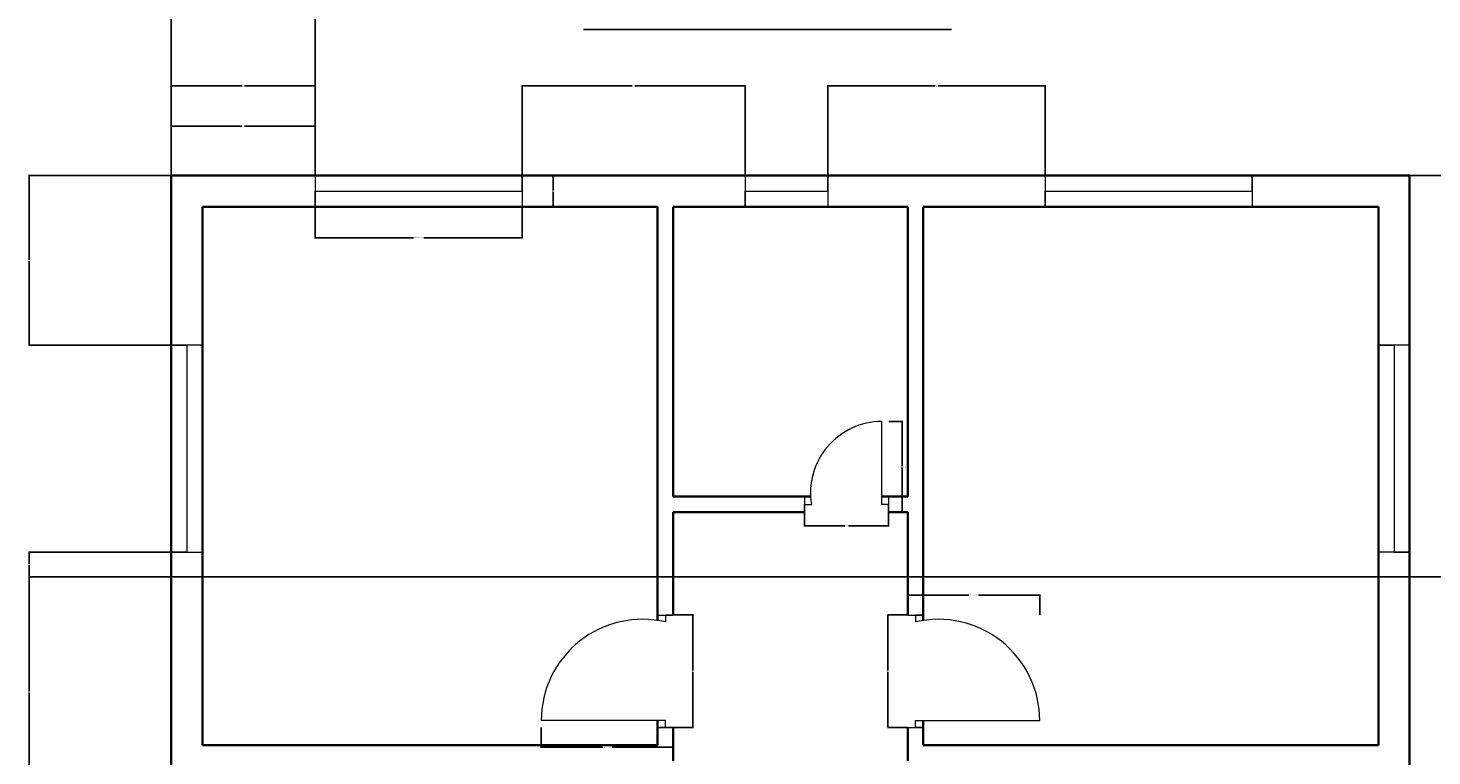
# Model space of a CAD drawing. Units: inches. Extents: x 1832 to 2989, y 1644 to 2902.
# Tile 5 of 8: x 2354 to 2760, y 2061 to 2272. Entities that reach past the tile are written whole.
import ezdxf

# ---------------------------------------------------------------- set-up
doc = ezdxf.new("R2010")
doc.units = ezdxf.units.IN
for name, color, linetype, lineweight in [('A-ANNO-DIMS', 2, 'Continuous', 18), ('A-ANNO-SYMB', 3, 'Continuous', 25), ('A-ANNO-TEXT', 7, 'Continuous', 25), ('A-DOOR', 3, 'Continuous', 18), ('A-GLAZ', 4, 'Continuous', 18), ('A-WALL', 7, 'Continuous', 35)]:
    doc.layers.add(name, color=color, linetype=linetype, lineweight=lineweight)
doc.styles.get("Standard").update_dxf_attribs({"font": 'arial.ttf'})
doc.dimstyles.get("Standard").update_dxf_attribs({"dimtxt": 0.18, "dimasz": 0.18, "dimexe": 0.18, "dimexo": 0.0625, "dimgap": 0.09, "dimtad": 0, "dimtih": 1, "dimtoh": 1, "dimdec": 4, "dimzin": 0, "dimdsep": 46, "dimtxsty": 'Standard', "dimcen": 0.09, "dimadec": 0, "dimazin": 0, "dimtfac": 1, "dimtdec": 4, "dimtofl": 0, "dimtmove": 0, "dimatfit": 3, "dimfxl": 1, "dimtolj": 1, "dimtzin": 0, "dimarcsym": 0})

# ---------------------------------------------------------------- blocks, each defined once
blk = doc.blocks.new('WIN-PLAN-60IN')
for p, q in [((0, 9), (0, 0)), ((60, 4.5), (60, 9)), ((60, 9), (60, 0)), ((0, 0), (0, 4.5)), ((0, 4.5), (60, 4.5))]:
    blk.add_line(p, q)
blk = doc.blocks.new('WIN-PLAN-60IN-2')
for p, q in [((9, 60), (0, 60)), ((0, 60), (4.5, 60)), ((4.5, 60), (4.5, 0)), ((4.5, 0), (0, 0)), ((0, 0), (9, 0))]:
    blk.add_line(p, q)
blk = doc.blocks.new('WIN-PLAN-24IN')
for p, q in [((0, 9), (0, 0)), ((24, 4.5), (24, 9)), ((24, 9), (24, 0)), ((0, 0), (0, 4.5)), ((0, 4.5), (24, 4.5))]:
    blk.add_line(p, q)
blk = doc.blocks.new('DOOR-PLAN-BEDROOM-L')
for p, q in [((33.75, 32.55), (38.25, 32.55)), ((38.25, 32.55), (36, 32.55)), ((36, 32.55), (36, 30.55)), ((36, 2), (0, 2)), ((33.75, 0), (38.25, 0)), ((38.25, 0), (33.75, 0)), ((33.75, 0), (36, 0)), ((36, 0), (36, 2))]:
    blk.add_line(p, q)
blk.add_arc((29.32, 2), 29.32, 76.8389, 180)
blk = doc.blocks.new('DOOR-PLAN-BATH')
for p, q in [((22.39, 2.25), (22.39, 26.25)), ((0, 4.5), (0, 0)), ((24.39, 4.5), (24.39, 0)), ((0, 0), (0, 2.25)), ((0, 2.25), (2, 2.25)), ((24.39, 2.25), (22.39, 2.25)), ((24.39, 0), (24.39, 2.25))]:
    blk.add_line(p, q)
blk.add_arc((22.39, 5.59), 20.66, 90, 189.2955)
blk = doc.blocks.new('DOOR-PLAN-BEDROOM-R')
for p, q in [((0, 32.55), (4.5, 32.55)), ((4.5, 32.55), (2.25, 32.55)), ((2.25, 32.55), (2.25, 30.55)), ((0, 0), (4.5, 0)), ((2.25, 0), (2.25, 2)), ((2.25, 2), (38.25, 2)), ((4.5, 0), (2.25, 0))]:
    blk.add_line(p, q)
blk.add_arc((8.93, 2), 29.32, 0, 103.1611)
blk = doc.blocks.new('*D37')
at = {"layer": 'A-ANNO-DIMS', "color": 0, "lineweight": -2, "transparency": 16777216}
for p, q in [((2502.29, 2069.25), (2502.29, 2063.39)), ((2540.54, 2069.25), (2540.54, 2063.39)), ((2502.47, 2063.57), (2520.01, 2063.57)), ((2540.36, 2063.57), (2522.81, 2063.57))]:
    blk.add_line(p, q, dxfattribs=at)
at = {"layer": 'A-ANNO-DIMS', "color": 0, "transparency": 16777216}
for points in [[(2502.47, 2063.6), (2502.47, 2063.54), (2502.29, 2063.57)], [(2540.36, 2063.6), (2540.36, 2063.54), (2540.54, 2063.57)]]:
    blk.add_solid(points, dxfattribs=at)
at = {"layer": 'Defpoints', "color": 0, "transparency": 16777216}
for p in [(2502.29, 2069.31), (2540.54, 2069.31), (2540.54, 2063.57)]:
    blk.add_point(p, dxfattribs=at)
at = {"layer": 'A-ANNO-DIMS', "color": 0, "transparency": 16777216, "insert": (2521.41, 2063.57), "char_height": 0.18, "attachment_point": 5}
blk.add_mtext('\\A1;BEDROOM LH 38 TYP.', dxfattribs=at)
blk = doc.blocks.new('*D38')
at = {"layer": 'A-ANNO-DIMS', "color": 0, "lineweight": -2, "transparency": 16777216}
for p, q in [((2540.6, 2101.9), (2546.45, 2101.9)), ((2546.27, 2101.72), (2546.27, 2085.79)), ((2546.27, 2069.49), (2546.27, 2085.43)), ((2540.6, 2069.31), (2546.45, 2069.31))]:
    blk.add_line(p, q, dxfattribs=at)
at = {"layer": 'A-ANNO-DIMS', "color": 0, "transparency": 16777216}
for points in [[(2546.24, 2101.72), (2546.3, 2101.72), (2546.27, 2101.9)], [(2546.24, 2069.49), (2546.3, 2069.49), (2546.27, 2069.31)]]:
    blk.add_solid(points, dxfattribs=at)
at = {"layer": 'Defpoints', "color": 0, "transparency": 16777216}
for p in [(2540.54, 2101.9), (2546.27, 2101.9), (2540.54, 2069.31)]:
    blk.add_point(p, dxfattribs=at)
at = {"layer": 'A-ANNO-DIMS', "color": 0, "transparency": 16777216, "insert": (2546.27, 2085.61), "char_height": 0.18, "attachment_point": 5}
blk.add_mtext('\\A1;33 TYP.', dxfattribs=at)
blk = doc.blocks.new('*D39')
at = {"layer": 'A-ANNO-DIMS', "color": 0, "lineweight": -2, "transparency": 16777216}
for p, q in [((2608.54, 2101.97), (2608.54, 2107.82)), ((2608.72, 2107.64), (2626.24, 2107.64)), ((2646.61, 2107.64), (2629.09, 2107.64)), ((2646.79, 2101.97), (2646.79, 2107.82))]:
    blk.add_line(p, q, dxfattribs=at)
at = {"layer": 'A-ANNO-DIMS', "color": 0, "transparency": 16777216}
for points in [[(2608.72, 2107.67), (2608.72, 2107.61), (2608.54, 2107.64)], [(2646.61, 2107.67), (2646.61, 2107.61), (2646.79, 2107.64)]]:
    blk.add_solid(points, dxfattribs=at)
at = {"layer": 'Defpoints', "color": 0, "transparency": 16777216}
for p in [(2646.79, 2107.64), (2608.54, 2101.9), (2646.79, 2101.9)]:
    blk.add_point(p, dxfattribs=at)
at = {"layer": 'A-ANNO-DIMS', "color": 0, "transparency": 16777216, "insert": (2627.66, 2107.64), "char_height": 0.18, "attachment_point": 5}
blk.add_mtext('\\A1;BEDROOM RH 38 TYP.', dxfattribs=at)
blk = doc.blocks.new('*D40')
at = {"layer": 'A-ANNO-DIMS', "color": 0, "lineweight": -2, "transparency": 16777216}
for p, q in [((2608.47, 2101.9), (2602.62, 2101.9)), ((2602.8, 2101.72), (2602.8, 2085.79)), ((2602.8, 2069.49), (2602.8, 2085.43)), ((2608.47, 2069.31), (2602.62, 2069.31))]:
    blk.add_line(p, q, dxfattribs=at)
at = {"layer": 'A-ANNO-DIMS', "color": 0, "transparency": 16777216}
for points in [[(2602.77, 2101.72), (2602.83, 2101.72), (2602.8, 2101.9)], [(2602.77, 2069.49), (2602.83, 2069.49), (2602.8, 2069.31)]]:
    blk.add_solid(points, dxfattribs=at)
at = {"layer": 'Defpoints', "color": 0, "transparency": 16777216}
for p in [(2602.8, 2101.9), (2608.54, 2101.9), (2608.54, 2069.31)]:
    blk.add_point(p, dxfattribs=at)
at = {"layer": 'A-ANNO-DIMS', "color": 0, "transparency": 16777216, "insert": (2602.8, 2085.61), "char_height": 0.18, "attachment_point": 5}
blk.add_mtext('\\A1;33 TYP.', dxfattribs=at)
blk = doc.blocks.new('*D41')
at = {"layer": 'A-ANNO-DIMS', "color": 0, "lineweight": -2, "transparency": 16777216}
for p, q in [((2603.06, 2157.92), (2607.12, 2157.92)), ((2606.94, 2157.74), (2606.94, 2144.98)), ((2606.94, 2131.85), (2606.94, 2144.61)), ((2603.06, 2131.67), (2607.12, 2131.67))]:
    blk.add_line(p, q, dxfattribs=at)
at = {"layer": 'A-ANNO-DIMS', "color": 0, "transparency": 16777216}
for points in [[(2606.91, 2157.74), (2606.97, 2157.74), (2606.94, 2157.92)], [(2606.91, 2131.85), (2606.97, 2131.85), (2606.94, 2131.67)]]:
    blk.add_solid(points, dxfattribs=at)
at = {"layer": 'Defpoints', "color": 0, "transparency": 16777216}
for p in [(2603, 2157.92), (2606.94, 2157.92), (2603, 2131.67)]:
    blk.add_point(p, dxfattribs=at)
at = {"layer": 'A-ANNO-DIMS', "color": 0, "transparency": 16777216, "insert": (2606.94, 2144.8), "char_height": 0.18, "attachment_point": 5}
blk.add_mtext('\\A1;BATH DOOR 26 TYP.', dxfattribs=at)
blk = doc.blocks.new('*D42')
at = {"layer": 'A-ANNO-DIMS', "color": 0, "lineweight": -2, "transparency": 16777216}
for p, q in [((2578.61, 2131.61), (2578.61, 2127.56)), ((2603, 2131.61), (2603, 2127.56)), ((2578.79, 2127.74), (2590.28, 2127.74)), ((2602.82, 2127.74), (2591.33, 2127.74))]:
    blk.add_line(p, q, dxfattribs=at)
at = {"layer": 'A-ANNO-DIMS', "color": 0, "transparency": 16777216}
for points in [[(2578.79, 2127.77), (2578.79, 2127.71), (2578.61, 2127.74)], [(2602.82, 2127.77), (2602.82, 2127.71), (2603, 2127.74)]]:
    blk.add_solid(points, dxfattribs=at)
at = {"layer": 'Defpoints', "color": 0, "transparency": 16777216}
for p in [(2578.61, 2131.67), (2603, 2131.67), (2603, 2127.74)]:
    blk.add_point(p, dxfattribs=at)
at = {"layer": 'A-ANNO-DIMS', "color": 0, "transparency": 16777216, "insert": (2590.81, 2127.74), "char_height": 0.18, "attachment_point": 5}
blk.add_mtext('\\A1;24 TYP.', dxfattribs=at)
blk = doc.blocks.new('*D49')
at = {"layer": 'A-ANNO-DIMS', "color": 0, "lineweight": -2, "transparency": 16777216}
for p, q in [((2436.72, 2220.11), (2436.72, 2210.99)), ((2496.72, 2220.11), (2496.72, 2210.99)), ((2436.9, 2211.17), (2465.22, 2211.17)), ((2496.54, 2211.17), (2468.21, 2211.17))]:
    blk.add_line(p, q, dxfattribs=at)
at = {"layer": 'A-ANNO-DIMS', "color": 0, "transparency": 16777216}
for points in [[(2436.9, 2211.2), (2436.9, 2211.14), (2436.72, 2211.17)], [(2496.54, 2211.2), (2496.54, 2211.14), (2496.72, 2211.17)]]:
    blk.add_solid(points, dxfattribs=at)
at = {"layer": 'Defpoints', "color": 0, "transparency": 16777216}
for p in [(2436.72, 2220.17), (2496.72, 2220.17), (2496.72, 2211.17)]:
    blk.add_point(p, dxfattribs=at)
at = {"layer": 'A-ANNO-DIMS', "color": 0, "transparency": 16777216, "insert": (2466.72, 2211.17), "char_height": 0.18, "attachment_point": 5}
blk.add_mtext('\\A1;REAR WINDOW 60 TYP.', dxfattribs=at)
blk = doc.blocks.new('*D50')
at = {"layer": 'A-ANNO-DIMS', "color": 0, "lineweight": -2, "transparency": 16777216}
for p, q in [((2496.78, 2229.17), (2505.9, 2229.17)), ((2505.72, 2228.99), (2505.72, 2224.85)), ((2505.72, 2220.35), (2505.72, 2224.49)), ((2496.78, 2220.17), (2505.9, 2220.17))]:
    blk.add_line(p, q, dxfattribs=at)
at = {"layer": 'A-ANNO-DIMS', "color": 0, "transparency": 16777216}
for points in [[(2505.69, 2228.99), (2505.75, 2228.99), (2505.72, 2229.17)], [(2505.69, 2220.35), (2505.75, 2220.35), (2505.72, 2220.17)]]:
    blk.add_solid(points, dxfattribs=at)
at = {"layer": 'Defpoints', "color": 0, "transparency": 16777216}
for p in [(2496.72, 2229.17), (2505.72, 2229.17), (2496.72, 2220.17)]:
    blk.add_point(p, dxfattribs=at)
at = {"layer": 'A-ANNO-DIMS', "color": 0, "transparency": 16777216, "insert": (2505.72, 2224.67), "char_height": 0.18, "attachment_point": 5}
blk.add_mtext('\\A1;9 TYP.', dxfattribs=at)
blk = doc.blocks.new('*D82')
at = {"layer": 'A-ANNO-DIMS', "color": 0, "lineweight": -2, "transparency": 16777216}
for p, q in [((2754.1, 2229.17), (2811, 2229.17)), ((2810.82, 2228.99), (2810.82, 1975.53)), ((2810.82, 1721.7), (2810.82, 1975.17)), ((2745.1, 1721.52), (2811, 1721.52))]:
    blk.add_line(p, q, dxfattribs=at)
at = {"layer": 'A-ANNO-DIMS', "color": 0, "transparency": 16777216}
for points in [[(2810.79, 2228.99), (2810.85, 2228.99), (2810.82, 2229.17)], [(2810.79, 1721.7), (2810.85, 1721.7), (2810.82, 1721.52)]]:
    blk.add_solid(points, dxfattribs=at)
at = {"layer": 'Defpoints', "color": 0, "transparency": 16777216}
for p in [(2754.04, 2229.17), (2810.82, 2229.17), (2745.04, 1721.52)]:
    blk.add_point(p, dxfattribs=at)
at = {"layer": 'A-ANNO-DIMS', "color": 0, "transparency": 16777216, "insert": (2810.82, 1975.35), "char_height": 0.18, "attachment_point": 5}
blk.add_mtext('\\A1;507.6', dxfattribs=at)
blk = doc.blocks.new('*D85')
at = {"layer": 'A-ANNO-DIMS', "color": 0, "lineweight": -2, "transparency": 16777216}
for p, q in [((2379.76, 2112.91), (2353.64, 2112.91)), ((2353.82, 2112.73), (2353.82, 2079.83)), ((2353.82, 2046.57), (2353.82, 2079.47)), ((2394.97, 2046.39), (2353.64, 2046.39))]:
    blk.add_line(p, q, dxfattribs=at)
at = {"layer": 'A-ANNO-DIMS', "color": 0, "transparency": 16777216}
for points in [[(2353.79, 2112.73), (2353.85, 2112.73), (2353.82, 2112.91)], [(2353.79, 2046.57), (2353.85, 2046.57), (2353.82, 2046.39)]]:
    blk.add_solid(points, dxfattribs=at)
at = {"layer": 'Defpoints', "color": 0, "transparency": 16777216}
for p in [(2353.82, 2112.91), (2379.82, 2112.91), (2395.04, 2046.39)]:
    blk.add_point(p, dxfattribs=at)
at = {"layer": 'A-ANNO-DIMS', "color": 0, "transparency": 16777216, "insert": (2353.82, 2079.65), "char_height": 0.18, "attachment_point": 5}
blk.add_mtext('\\A1;66.53', dxfattribs=at)
blk = doc.blocks.new('*D86')
at = {"layer": 'A-ANNO-DIMS', "color": 0, "lineweight": -2, "transparency": 16777216}
for p, q in [((2394.97, 2120.08), (2353.64, 2120.08)), ((2353.82, 2119.9), (2353.82, 2116.68)), ((2379.76, 2112.91), (2353.64, 2112.91)), ((2353.82, 2113.09), (2353.82, 2116.32))]:
    blk.add_line(p, q, dxfattribs=at)
at = {"layer": 'A-ANNO-DIMS', "color": 0, "transparency": 16777216}
for points in [[(2353.79, 2119.9), (2353.85, 2119.9), (2353.82, 2120.08)], [(2353.79, 2113.09), (2353.85, 2113.09), (2353.82, 2112.91)]]:
    blk.add_solid(points, dxfattribs=at)
at = {"layer": 'Defpoints', "color": 0, "transparency": 16777216}
for p in [(2353.82, 2120.08), (2395.04, 2120.08), (2379.82, 2112.91)]:
    blk.add_point(p, dxfattribs=at)
at = {"layer": 'A-ANNO-DIMS', "color": 0, "transparency": 16777216, "insert": (2353.82, 2116.5), "char_height": 0.18, "attachment_point": 5}
blk.add_mtext('\\A1;7.174', dxfattribs=at)
blk = doc.blocks.new('*D87')
at = {"layer": 'A-ANNO-DIMS', "color": 0, "lineweight": -2, "transparency": 16777216}
for p, q in [((2394.97, 2229.17), (2353.64, 2229.17)), ((2353.82, 2228.99), (2353.82, 2204.81)), ((2353.82, 2180.26), (2353.82, 2204.45)), ((2394.97, 2180.08), (2353.64, 2180.08))]:
    blk.add_line(p, q, dxfattribs=at)
at = {"layer": 'A-ANNO-DIMS', "color": 0, "transparency": 16777216}
for points in [[(2353.79, 2228.99), (2353.85, 2228.99), (2353.82, 2229.17)], [(2353.79, 2180.26), (2353.85, 2180.26), (2353.82, 2180.08)]]:
    blk.add_solid(points, dxfattribs=at)
at = {"layer": 'Defpoints', "color": 0, "transparency": 16777216}
for p in [(2353.82, 2229.17), (2395.04, 2229.17), (2395.04, 2180.08)]:
    blk.add_point(p, dxfattribs=at)
at = {"layer": 'A-ANNO-DIMS', "color": 0, "transparency": 16777216, "insert": (2353.82, 2204.63), "char_height": 0.18, "attachment_point": 5}
blk.add_mtext('\\A1;49.09', dxfattribs=at)
blk = doc.blocks.new('*D88')
at = {"layer": 'A-ANNO-DIMS', "color": 0, "lineweight": -2, "transparency": 16777216}
for p, q in [((2395.04, 2229.24), (2395.04, 2255.35)), ((2395.22, 2255.17), (2415.48, 2255.17)), ((2436.54, 2255.17), (2416.27, 2255.17)), ((2436.72, 2229.24), (2436.72, 2255.35))]:
    blk.add_line(p, q, dxfattribs=at)
at = {"layer": 'A-ANNO-DIMS', "color": 0, "transparency": 16777216}
for points in [[(2395.22, 2255.2), (2395.22, 2255.14), (2395.04, 2255.17)], [(2436.54, 2255.2), (2436.54, 2255.14), (2436.72, 2255.17)]]:
    blk.add_solid(points, dxfattribs=at)
at = {"layer": 'Defpoints', "color": 0, "transparency": 16777216}
for p in [(2436.72, 2255.17), (2395.04, 2229.17), (2436.72, 2229.17)]:
    blk.add_point(p, dxfattribs=at)
at = {"layer": 'A-ANNO-DIMS', "color": 0, "transparency": 16777216, "insert": (2415.88, 2255.17), "char_height": 0.18, "attachment_point": 5}
blk.add_mtext('\\A1;41.68', dxfattribs=at)
blk = doc.blocks.new('*D89')
at = {"layer": 'A-ANNO-DIMS', "color": 0, "lineweight": -2, "transparency": 16777216}
for p, q in [((2496.72, 2229.24), (2496.72, 2255.35)), ((2496.9, 2255.17), (2528.64, 2255.17)), ((2561.18, 2255.17), (2529.43, 2255.17)), ((2561.36, 2229.24), (2561.36, 2255.35))]:
    blk.add_line(p, q, dxfattribs=at)
at = {"layer": 'A-ANNO-DIMS', "color": 0, "transparency": 16777216}
for points in [[(2496.9, 2255.2), (2496.9, 2255.14), (2496.72, 2255.17)], [(2561.18, 2255.2), (2561.18, 2255.14), (2561.36, 2255.17)]]:
    blk.add_solid(points, dxfattribs=at)
at = {"layer": 'Defpoints', "color": 0, "transparency": 16777216}
for p in [(2561.36, 2255.17), (2496.72, 2229.17), (2561.36, 2229.17)]:
    blk.add_point(p, dxfattribs=at)
at = {"layer": 'A-ANNO-DIMS', "color": 0, "transparency": 16777216, "insert": (2529.04, 2255.17), "char_height": 0.18, "attachment_point": 5}
blk.add_mtext('\\A1;64.64', dxfattribs=at)
blk = doc.blocks.new('*D90')
at = {"layer": 'A-ANNO-DIMS', "color": 0, "lineweight": -2, "transparency": 16777216}
for p, q in [((2585.36, 2229.24), (2585.36, 2255.35)), ((2585.54, 2255.17), (2616.48, 2255.17)), ((2648.21, 2255.17), (2617.27, 2255.17)), ((2648.39, 2229.24), (2648.39, 2255.35))]:
    blk.add_line(p, q, dxfattribs=at)
at = {"layer": 'A-ANNO-DIMS', "color": 0, "transparency": 16777216}
for points in [[(2585.54, 2255.2), (2585.54, 2255.14), (2585.36, 2255.17)], [(2648.21, 2255.2), (2648.21, 2255.14), (2648.39, 2255.17)]]:
    blk.add_solid(points, dxfattribs=at)
at = {"layer": 'Defpoints', "color": 0, "transparency": 16777216}
for p in [(2648.39, 2255.17), (2585.36, 2229.17), (2648.39, 2229.17)]:
    blk.add_point(p, dxfattribs=at)
at = {"layer": 'A-ANNO-DIMS', "color": 0, "transparency": 16777216, "insert": (2616.87, 2255.17), "char_height": 0.18, "attachment_point": 5}
blk.add_mtext('\\A1;63.03', dxfattribs=at)
blk = doc.blocks.new('*D115')
at = {"layer": 'A-ANNO-DIMS', "color": 0, "lineweight": -2, "transparency": 16777216}
for p, q in [((2436.72, 2360.25), (2436.72, 2243.31)), ((2395.04, 2306.25), (2395.04, 2243.31)), ((2395.22, 2243.49), (2415.48, 2243.49)), ((2436.54, 2243.49), (2416.27, 2243.49))]:
    blk.add_line(p, q, dxfattribs=at)
at = {"layer": 'A-ANNO-DIMS', "color": 0, "transparency": 16777216}
for points in [[(2395.22, 2243.52), (2395.22, 2243.46), (2395.04, 2243.49)], [(2436.54, 2243.52), (2436.54, 2243.46), (2436.72, 2243.49)]]:
    blk.add_solid(points, dxfattribs=at)
at = {"layer": 'Defpoints', "color": 0, "transparency": 16777216}
for p in [(2436.72, 2360.31), (2395.04, 2306.31), (2436.72, 2243.49)]:
    blk.add_point(p, dxfattribs=at)
at = {"layer": 'A-ANNO-DIMS', "color": 0, "transparency": 16777216, "insert": (2415.88, 2243.49), "char_height": 0.18, "attachment_point": 5}
blk.add_mtext('\\A1;41.68', dxfattribs=at)

msp = doc.modelspace()

# ---------------------------------------------------------------- linework, layer by layer
at = {"layer": 'A-ANNO-SYMB'}
msp.add_line((2379.819, 2112.9108), (2784.8213, 2112.9108), dxfattribs=at)
at = {"layer": 'A-ANNO-TEXT'}
msp.add_line((2514.498, 2271.5366), (2621.2451, 2271.5366), dxfattribs=at)
at = {"layer": 'A-WALL'}
for p, q in [((2395.0354, 2229.1726), (2395.0354, 1750.6726)), ((2395.0354, 2229.1726), (2395.0354, 1750.6726)), ((2395.0354, 2229.1726), (2395.0354, 1750.6726)), ((2395.0354, 2229.1726), (2754.0354, 2229.1726)), ((2754.0354, 2229.1726), (2754.0354, 1846.6726)), ((2404.0354, 2220.1726), (2404.0354, 2064.1726)), ((2404.0354, 2220.1726), (2536.0354, 2220.1726)), ((2536.0354, 2220.1726), (2536.0354, 2100.2994)), ((2540.5354, 2220.1726), (2540.5354, 2136.1726)), ((2540.5354, 2220.1726), (2608.5354, 2220.1726)), ((2608.5354, 2220.1726), (2608.5354, 2136.1726)), ((2613.0354, 2220.1726), (2613.0354, 2100.2994)), ((2613.0354, 2220.1726), (2745.0354, 2220.1726)), ((2745.0354, 2220.1726), (2745.0354, 2064.1726)), ((2540.5354, 2136.1726), (2580.3671, 2136.1726)), ((2601.0009, 2136.1726), (2608.5354, 2136.1726)), ((2540.5354, 2131.6726), (2540.5354, 2101.8652)), ((2540.5354, 2131.6726), (2578.6098, 2131.6726)), ((2603.0009, 2131.6726), (2608.5354, 2131.6726)), ((2608.5354, 2131.6726), (2608.5354, 2101.8652)), ((2536.0354, 2071.312), (2536.0354, 2064.1726)), ((2540.5354, 2069.312), (2540.5354, 2064.1726)), ((2608.5354, 2069.312), (2608.5354, 2064.1726)), ((2613.0354, 2071.312), (2613.0354, 2064.1726)), ((2404.0354, 2064.1726), (2536.0354, 2064.1726)), ((2540.5354, 2064.1726), (2540.5354, 2059.6726)), ((2608.5354, 2064.1726), (2608.5354, 2059.6726)), ((2613.0354, 2064.1726), (2745.0354, 2064.1726))]:
    msp.add_line(p, q, dxfattribs=at)

# ---------------------------------------------------------------- block references
at = {"layer": 'A-DOOR'}
for name, p in [('DOOR-PLAN-BATH', (2578.6098, 2131.6726)), ('DOOR-PLAN-BEDROOM-L', (2502.2854, 2069.312)), ('DOOR-PLAN-BEDROOM-R', (2608.5354, 2069.312))]:
    msp.add_blockref(name, p, dxfattribs=at)
at = {"layer": 'A-GLAZ'}
for name, p in [('WIN-PLAN-60IN', (2436.7169, 2220.1726)), ('WIN-PLAN-24IN', (2561.3579, 2220.1726)), ('WIN-PLAN-60IN', (2648.3901, 2220.1726)), ('WIN-PLAN-60IN-2', (2395.0354, 2120.0845))]:
    msp.add_blockref(name, p, dxfattribs=at)
at = {"layer": 'A-GLAZ', "rotation": 269.9999999999992}
msp.add_blockref('WIN-PLAN-60IN', (2745.0354, 2180.0845), dxfattribs=at)

# ---------------------------------------------------------------- dimensions: what is measured, and where the dimension line sits
at = {"layer": 'A-ANNO-DIMS'}
for base, p1, p2, picture, middle in [((2436.7169, 2243.4866), (2395.0354, 2306.3121), (2436.7169, 2360.3121), '*D115', (2415.8762, 2243.4866)), ((2436.7169, 2255.1726), (2395.0354, 2229.1726), (2436.7169, 2229.1726), '*D88', (2415.8762, 2255.1726)), ((2561.3579, 2255.1726), (2496.7169, 2229.1726), (2561.3579, 2229.1726), '*D89', (2529.0374, 2255.1726)), ((2648.3901, 2255.1726), (2585.3579, 2229.1726), (2648.3901, 2229.1726), '*D90', (2616.874, 2255.1726))]:
    dim = msp.add_linear_dim(base=base, p1=p1, p2=p2, dimstyle='Standard', override={"dimdec": 2, "dimlfac": 1, "dimrnd": 0, "dimzin": 0, "dimdsep": 46, "dimlunit": 2}, dxfattribs=at)
    dim.commit()
    dim.dimension.update_dxf_attribs({"geometry": picture, "text_midpoint": middle})
for base, p1, p2, override, picture, middle in [((2353.819, 2229.1726), (2395.0354, 2180.0845), (2395.0354, 2229.1726), {"dimdec": 2, "dimlfac": 1, "dimrnd": 0, "dimzin": 0, "dimdsep": 46, "dimlunit": 2}, '*D87', (2353.819, 2204.6285)), ((2810.8213, 2229.1726), (2745.0354, 1721.5243), (2754.0354, 2229.1726), {"dimdec": 1, "dimlfac": 1, "dimrnd": 0, "dimzin": 0, "dimdsep": 46, "dimlunit": 2}, '*D82', (2810.8213, 1975.3484)), ((2353.819, 2120.0845), (2379.819, 2112.9108), (2395.0354, 2120.0845), {"dimdec": 3, "dimlfac": 1, "dimrnd": 0, "dimzin": 0, "dimdsep": 46, "dimlunit": 2}, '*D86', (2353.819, 2116.4976)), ((2353.819, 2112.9108), (2395.0354, 2046.3857), (2379.819, 2112.9108), {"dimdec": 2, "dimlfac": 1, "dimrnd": 0, "dimzin": 0, "dimdsep": 46, "dimlunit": 2}, '*D85', (2353.819, 2079.6483))]:
    dim = msp.add_linear_dim(base=base, p1=p1, p2=p2, angle=90, dimstyle='Standard', override=override, dxfattribs=at)
    dim.commit()
    dim.dimension.update_dxf_attribs({"geometry": picture, "text_midpoint": middle})
for base, p1, p2, text, picture, middle in [((2505.7169, 2229.1726), (2496.7169, 2220.1726), (2496.7169, 2229.1726), '<> TYP.', '*D50', (2505.7169, 2224.6726)), ((2606.9384, 2157.9226), (2603.0009, 2131.6726), (2603.0009, 2157.9226), 'BATH DOOR <> TYP.', '*D41', (2606.9384, 2144.7976)), ((2546.2729, 2101.9033), (2540.5354, 2069.312), (2540.5354, 2101.9033), '<> TYP.', '*D38', (2546.2729, 2085.6077)), ((2602.7979, 2101.9033), (2608.5354, 2069.312), (2608.5354, 2101.9033), '<> TYP.', '*D40', (2602.7979, 2085.6077))]:
    dim = msp.add_linear_dim(base=base, p1=p1, p2=p2, angle=90, text=text, dimstyle='Standard', override={"dimdec": 0, "dimlfac": 1, "dimrnd": 0, "dimzin": 0, "dimdsep": 46, "dimlunit": 2}, dxfattribs=at)
    dim.commit()
    dim.dimension.update_dxf_attribs({"geometry": picture, "text_midpoint": middle})
for base, p1, p2, text, picture, middle in [((2496.7169, 2211.1726), (2436.7169, 2220.1726), (2496.7169, 2220.1726), 'REAR WINDOW <> TYP.', '*D49', (2466.7169, 2211.1726)), ((2603.0009, 2127.7351), (2578.6098, 2131.6726), (2603.0009, 2131.6726), '<> TYP.', '*D42', (2590.8054, 2127.7351)), ((2646.7854, 2107.6408), (2608.5354, 2101.9033), (2646.7854, 2101.9033), 'BEDROOM RH <> TYP.', '*D39', (2627.6604, 2107.6408)), ((2540.5354, 2063.5745), (2502.2854, 2069.312), (2540.5354, 2069.312), 'BEDROOM LH <> TYP.', '*D37', (2521.4104, 2063.5745))]:
    dim = msp.add_linear_dim(base=base, p1=p1, p2=p2, text=text, dimstyle='Standard', override={"dimdec": 0, "dimlfac": 1, "dimrnd": 0, "dimzin": 0, "dimdsep": 46, "dimlunit": 2}, dxfattribs=at)
    dim.commit()
    dim.dimension.update_dxf_attribs({"geometry": picture, "text_midpoint": middle})

doc.saveas('drawing.dxf')
